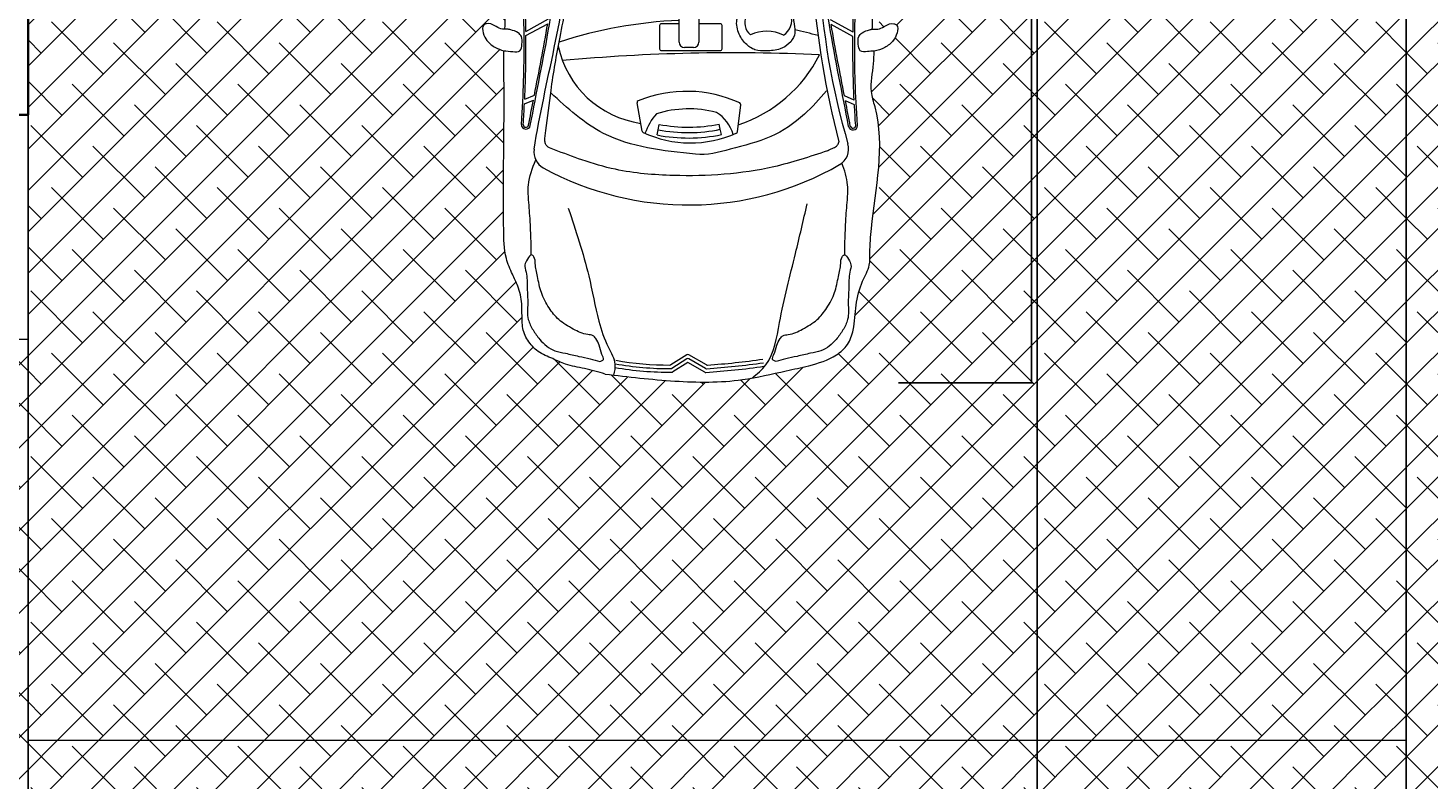
# Model space of a CAD drawing. Units: inches. Extents: x -4843 to -3402, y -164 to 3629.
# Tile 3 of 22: x -4303 to -3999, y 131 to 294. Entities that reach past the tile are written whole.
import ezdxf

# ---------------------------------------------------------------- set-up
doc = ezdxf.new("R2010")
doc.units = ezdxf.units.IN
for name, color, linetype, lineweight in [('A-ANNO-DIMS', 2, 'Continuous', 18), ('C-PRKG-VEHI', 7, 'Continuous', 18), ('C-PVMT', 7, 'Continuous', 18), ('walls', 7, 'Continuous', 35)]:
    doc.layers.add(name, color=color, linetype=linetype, lineweight=lineweight)
doc.layers.add('C-PVMT-PATT', color=9, linetype='Continuous', lineweight=13, true_color=0xc7c8ca)
doc.styles.get("Standard").update_dxf_attribs({"font": 'arial.ttf'})
doc.dimstyles.get("Standard").update_dxf_attribs({"dimtxt": 0.18, "dimasz": 0.18, "dimexe": 0.18, "dimexo": 0.0625, "dimgap": 0.09, "dimtad": 0, "dimtih": 1, "dimtoh": 1, "dimdec": 4, "dimzin": 0, "dimdsep": 46, "dimtxsty": 'Standard', "dimcen": 0.09, "dimadec": 0, "dimazin": 0, "dimtfac": 1, "dimtdec": 4, "dimtofl": 0, "dimtmove": 0, "dimatfit": 3, "dimfxl": 1, "dimtolj": 1, "dimtzin": 0, "dimarcsym": 0})
pattern_1 = [(45, (-7766.296, -1992.247), (-4.490128, 4.490128), []), (135, (-7766.296, -1992.247), (-13.470384, 4.490128), [15.875, -9.525])]

# ---------------------------------------------------------------- blocks, each defined once
blk = doc.blocks.new('A$C3DA776D3')
for p, q in [((1.3708, 1.8398), (1.39, 1.7957)), ((1.3941, 1.8386), (1.4148, 1.7908)), ((1.7076, 1.8326), (1.7664, 1.7249)), ((1.7285, 1.8328), (1.7896, 1.7211)), ((1.2367, 1.2599), (1.3767, 1.2842)), ((1.2178, 1.1855), (1.2439, 1.1804)), ((1.2439, 1.1804), (1.27, 1.1752)), ((0.0962, 1.0335), (0.0497, 1.1077)), ((0.114, 1.0384), (0.0674, 1.1128)), ((0.1347, 1.0387), (0.0852, 1.1179)), ((1.6488, 1.0062), (1.6488, 1.051)), ((1.6754, 1.0776), (1.84, 1.0776)), ((0.0487, 0.9511), (0.0962, 1.0335)), ((0.0668, 0.9469), (0.1142, 1.0292)), ((0.0848, 0.9427), (0.1349, 1.0296)), ((1.8376, 0.9796), (1.6754, 0.9796)), ((1.2197, 0.8688), (1.2457, 0.8743)), ((1.2457, 0.8743), (1.2717, 0.8798)), ((1.2339, 0.7901), (1.3663, 0.7728)), ((1.7032, 0.2201), (1.7621, 0.3277)), ((1.7242, 0.2199), (1.7853, 0.3316)), ((1.3665, 0.2129), (1.3856, 0.257)), ((1.3897, 0.2141), (1.4105, 0.2619))]:
    blk.add_line(p, q)
blk.add_lwpolyline([(1.7676, 0.9796), (1.7676, 0.876, -0.414214), (1.7587, 0.8671), (1.6411, 0.8671, -0.414214), (1.6323, 0.876), (1.6323, 1.1626, -0.414214), (1.6411, 1.1715), (1.7587, 1.1715, -0.414214), (1.7676, 1.1626), (1.7676, 1.0776)], format="xyb")
for centre, radius, start, end in [((1.2688, 1.8326), 0.0222, 88.30081, 259.23573), ((1.2688, 1.8326), 0.0133, 88.30081, 259.23573), ((2.3634, 1.0306), 1.4908, 151.27714, 209.97599), ((1.1337, 1.7044), 0.0887, 80.92793, 151.27714), ((1.7558, 1.1977), 0.4855, 101.85595, 171.84728), ((-0.4678, 0.9763), 2.2529, 2.57809, 17.91043), ((-7.7929, 0.8063), 9.4158, 357.43424, 5.15957), ((1.6427, 1.1201), 1.5944, 170.12112, 180.27968), ((1.6427, 1.1201), 1.5767, 170.06503, 180.09581), ((1.6427, 1.1201), 1.5589, 170.06503, 179.90871), ((1.7341, 1.0216), 0.5553, 155.15631, 204.0455), ((1.1185, 0.9515), 0.313, 49.40393, 69.93973), ((1.2382, 1.2512), 0.00887, 99.85481, 155.15631), ((0.8039, 1.0409), 0.6292, 335.29473, 22.22123), ((1.3782, 1.2755), 0.00887, 22.22123, 99.85481), ((1.9963, 1.0318), 0.7935, 168.82603, 191.84879), ((1.9963, 1.0318), 0.7669, 168.82603, 191.84879), ((1.9963, 1.0318), 0.7403, 168.82603, 191.84879), ((0.8099, 1.0292), 0.5366, 345.36448, 17.33436), ((0.0572, 1.1124), 0.00887, 180.27968, 212.03468), ((0.075, 1.1175), 0.00887, 180.09581, 212.03468), ((0.0927, 1.1226), 0.00887, 179.90871, 212.03468), ((0.1065, 1.0337), 0.00887, 330.07292, 32.03468), ((0.1272, 1.034), 0.00887, 330.07292, 32.03468), ((1.6754, 1.051), 0.0266, 90, 180), ((1.6754, 1.0062), 0.0266, 180, 270), ((0.0564, 0.9467), 0.00887, 150.07292, 183.67668), ((3.6022, 1.1745), 3.562, 183.67668, 188.32383), ((0.0745, 0.9425), 0.00887, 150.07292, 183.76336), ((3.6022, 1.1745), 3.5442, 183.76336, 188.32383), ((0.0925, 0.9383), 0.00887, 150.07292, 183.85072), ((3.6022, 1.1745), 3.5265, 183.85072, 188.32383), ((1.1715, 0.9872), 0.1833, 285.46201, 329.30509), ((1.235, 0.7989), 0.00887, 204.0455, 262.57695), ((1.9221, 0.9991), 0.6875, 198.09737, 243.3215), ((1.3675, 0.7816), 0.00887, 262.57695, 335.29473), ((1.5443, 0.6456), 0.1854, 333.48481, 25.53467), ((1.7703, 0.6782), 0.0753, 62.21447, 141.10294), ((1.782, 0.6059), 0.0837, 210.97226, 288.84464), ((-0.4678, 0.9763), 2.2529, 344.97, 347.97913), ((2.3306, -4.2069), 4.6409, 94.71361, 104.29398), ((2.1977, -3.2479), 3.6398, 93.02386, 106.34052), ((1.1488, 0.33), 0.0887, 209.97599, 286.34052), ((1.1826, 0.2989), 0.00887, 252.27428, 284.29398), ((1.2645, 0.2201), 0.0222, 100.76427, 271.69919), ((1.2645, 0.2201), 0.0133, 100.76427, 271.69919)]:
    blk.add_arc(centre, radius, start, end)
for points, knots in [([(1.633, 1.9421), (1.6372, 1.9559), (1.6485, 1.9865), (1.6785, 2.0254), (1.7174, 2.0443), (1.758, 2.0499), (1.7712, 2.0175), (1.7589, 1.9877), (1.737, 1.958), (1.7418, 1.929), (1.7342, 1.9007), (1.7274, 1.874), (1.7007, 1.849), (1.6682, 1.8516), (1.625, 1.8563), (1.6294, 1.9016), (1.6314, 1.9281), (1.633, 1.9421)], [0.0885943, 0.0885943, 0.0885943, 0.0885943, 0.1373899, 0.1989553, 0.2458559, 0.2904509, 0.3067594, 0.3537167, 0.3919221, 0.4272917, 0.447055, 0.4910496, 0.5184931, 0.5619515, 0.6001709, 0.6402891, 0.6890715, 0.6890715, 0.6890715, 0.6890715]), ([(0.0396, 1.4417), (0.0491, 1.4755), (0.0673, 1.5404), (0.0818, 1.6302), (0.1179, 1.7036), (0.1448, 1.7742), (0.1943, 1.8176), (0.2482, 1.8478), (0.3113, 1.8529), (0.3899, 1.8505), (0.4662, 1.8663), (0.5364, 1.9021), (0.6273, 1.9413), (0.825, 1.9427), (1.0734, 1.9431), (1.3668, 1.9392), (1.5418, 1.9411), (1.633, 1.9421)], [0, 0, 0, 0, 0.118823, 0.228347, 0.304709, 0.395218, 0.479661, 0.520666, 0.602694, 0.688012, 0.788383, 0.860898, 0.954729, 1.11959, 1.518327, 1.801929, 2.110556, 2.110556, 2.110556, 2.110556]), ([(1.7401, 1.9359), (1.7441, 1.9358), (1.8578, 1.931), (2.1105, 1.9445), (2.4984, 1.9427), (2.8874, 1.9396), (3.2079, 1.9402), (3.5092, 1.9401), (3.7388, 1.9191), (3.9196, 1.945), (3.9792, 1.9134), (4.0141, 1.8916), (4.0511, 1.8608), (4.0944, 1.8389), (4.1316, 1.8213), (4.1705, 1.8314), (4.2164, 1.8107), (4.2677, 1.7817), (4.3166, 1.7281), (4.3472, 1.6107), (4.3777, 1.4199), (4.3756, 1.126), (4.3499, 0.8209), (4.3562, 0.5655), (4.3432, 0.4036), (4.2994, 0.3183), (4.2485, 0.2679), (4.1835, 0.2317), (4.102, 0.2378), (4.0429, 0.19), (3.9911, 0.1682), (3.96, 0.1386), (3.7692, 0.1231), (3.5761, 0.125), (3.3929, 0.1252), (3.3707, 0.1253)], [0.114046, 0.114046, 0.114046, 0.114046, 0.127519, 0.499235, 0.968453, 1.440308, 1.814622, 2.054514, 2.455224, 2.610949, 2.635875, 2.681833, 2.750323, 2.797084, 2.847368, 2.883024, 2.926275, 3.011124, 3.084414, 3.16311, 3.41524, 3.739789, 4.152943, 4.449449, 4.607544, 4.693588, 4.767288, 4.84799, 4.936972, 5.028501, 5.093159, 5.12765, 5.168553, 5.718196, 5.794044, 5.794044, 5.794044, 5.794044]), ([(0.1019, 1.4686), (0.1062, 1.4841), (0.1156, 1.5181), (0.1267, 1.5748), (0.1418, 1.6322), (0.1526, 1.7039), (0.1991, 1.7596), (0.2557, 1.7978), (0.3143, 1.8295), (0.3862, 1.8206), (0.4642, 1.8281), (0.5263, 1.8249), (0.5774, 1.8421), (0.6026, 1.8255), (0.6352, 1.809), (0.6121, 1.7865), (0.5738, 1.7879), (0.515, 1.7735), (0.4383, 1.7603), (0.3668, 1.7216), (0.3014, 1.6709), (0.2619, 1.6015), (0.2328, 1.5457), (0.2321, 1.5021), (0.2099, 1.4834), (0.1779, 1.4679), (0.1449, 1.4643), (0.1093, 1.4427), (0.1042, 1.4606), (0.1019, 1.4686)], [0, 0, 0, 0, 0.048183, 0.105687, 0.173148, 0.226645, 0.320656, 0.377708, 0.433539, 0.514499, 0.587235, 0.668333, 0.704408, 0.73448, 0.764541, 0.77911, 0.812729, 0.87811, 0.959931, 1.044551, 1.119493, 1.20463, 1.28096, 1.307559, 1.326943, 1.363733, 1.411478, 1.437083, 1.45761, 1.45761, 1.45761, 1.45761]), ([(0.6291, 1.8062), (0.6836, 1.8072), (0.7737, 1.8088), (0.887, 1.8185), (0.9906, 1.8256), (1.0541, 1.8003), (1.0947, 1.7841)], [0, 0, 0, 0, 0.1633136, 0.269827, 0.3423859, 0.4712329, 0.4712329, 0.4712329, 0.4712329]), ([(1.2647, 1.8108), (1.5866, 1.75), (1.9321, 1.6711), (2.357, 1.6555), (2.4305, 1.6528), (2.5038, 1.6481)], [0.0116221, 0.0116221, 0.0116221, 0.0116221, 0.1543947, 0.1543947, 0.1841997, 0.1841997, 0.1841997, 0.1841997]), ([(1.2695, 1.8548), (1.4293, 1.844), (1.6772, 1.8374), (2.0858, 1.8517), (2.5501, 1.8477), (2.9741, 1.8297), (3.2389, 1.8174), (3.3308, 1.8077), (3.7511, 1.7597)], [0.04998, 0.04998, 0.04998, 0.04998, 0.456658, 0.88886, 1.432548, 2.02833, 2.31987, 2.336539, 2.336539, 2.336539, 2.336539]), ([(1.3941, 1.8386), (1.4513, 1.8358), (1.5039, 1.8341), (1.6065, 1.8322), (1.6573, 1.8322), (1.7076, 1.8326)], [0.1630874, 0.1630874, 0.1630874, 0.1630874, 0.3282058, 0.3282058, 0.4985864, 0.4985864, 0.4985864, 0.4985864]), ([(1.7285, 1.8328), (1.7747, 1.8334), (1.8206, 1.8343), (1.9706, 1.8377), (2.0741, 1.8401), (2.2558, 1.8407), (2.3339, 1.8401), (2.412, 1.8388)], [0.5222333, 0.5222333, 0.5222333, 0.5222333, 0.6789211, 0.6789211, 1.0296365, 1.0296365, 1.2940564, 1.2940564, 1.2940564, 1.2940564]), ([(1.1452, 1.6917), (1.1484, 1.7027), (1.1532, 1.7193), (1.17, 1.7359), (1.1994, 1.7411), (1.2882, 1.7262), (1.4597, 1.7082), (1.664, 1.6726), (1.8239, 1.6391), (1.9094, 1.627), (1.9434, 1.6262), (1.9633, 1.6236), (1.9429, 1.5472), (1.9237, 1.3694), (1.9156, 1.0748), (1.9104, 0.7612), (1.9305, 0.5688), (1.9526, 0.4525), (1.9572, 0.4288)], [0, 0, 0, 0, 0.038062, 0.057765, 0.075887, 0.136118, 0.360736, 0.660851, 0.833831, 0.919425, 0.944413, 0.95681, 0.976133, 1.15453, 1.659168, 1.908025, 2.226872, 2.308645, 2.308645, 2.308645, 2.308645]), ([(1.1477, 1.792), (1.4905, 1.7373), (1.7995, 1.6413), (2.2125, 1.6082), (2.2832, 1.6032), (2.2832, 1.6032)], [0.0003636, 0.0003636, 0.0003636, 0.0003636, 0.134701, 0.134701, 0.1508358, 0.1508358, 0.1508358, 0.1508358]), ([(1.1396, 0.3464), (1.1105, 0.4339), (1.0553, 0.5995), (1.019, 0.8559), (1.0138, 1.1174), (1.0332, 1.3547), (1.0902, 1.5485), (1.1279, 1.6467), (1.1452, 1.6917)], [0, 0, 0, 0, 0.276247, 0.522812, 0.772814, 1.060937, 1.232089, 1.37667, 1.37667, 1.37667, 1.37667]), ([(1.1227, 0.9968), (1.1398, 1.1559), (1.169, 1.4274), (1.3493, 1.6278), (1.4252, 1.7102)], [0, 0, 0, 0, 0.5236809, 0.8940297, 0.8940297, 0.8940297, 0.8940297]), ([(0.857, 1.6234), (0.7466, 1.5866), (0.5639, 1.5256), (0.3275, 1.4841), (0.1848, 1.438), (0.1003, 1.3859), (0.0525, 1.3961), (0.0346, 1.4)], [0, 0, 0, 0, 0.3490723, 0.577526, 0.7150863, 0.8038491, 0.8574249, 0.8574249, 0.8574249, 0.8574249]), ([(0.0396, 1.4417), (0.0259, 1.3277), (-0.001, 1.1032), (-0.0041, 0.801), (0.0486, 0.5837), (0.0809, 0.4273), (0.1148, 0.3191), (0.1818, 0.2415), (0.2711, 0.2106), (0.3792, 0.2096), (0.4873, 0.1821), (0.5671, 0.1351), (0.6573, 0.1377), (0.9147, 0.1185), (1.1883, 0.0534), (1.4506, 0.141), (1.5438, 0.1176), (1.6105, 0.116), (1.6314, 0.1164)], [0, 0, 0, 0, 0.388807, 0.765455, 1.01322, 1.141907, 1.30735, 1.390473, 1.477778, 1.61655, 1.755196, 1.851534, 1.920565, 2.05458, 2.731843, 2.819344, 2.97386, 3.044752, 3.044752, 3.044752, 3.044752]), ([(1.4353, 0.3505), (1.3953, 0.3854), (1.3056, 0.4639), (1.1968, 0.6245), (1.1532, 0.8126), (1.1151, 0.9395), (1.1227, 0.9968)], [0, 0, 0, 0, 0.1591256, 0.357512, 0.5668997, 0.7404451, 0.7404451, 0.7404451, 0.7404451]), ([(1.8119, 0.5169), (1.7917, 0.514), (1.7583, 0.5092), (1.7058, 0.5035), (1.6658, 0.5348), (1.6354, 0.5836), (1.6317, 0.6432), (1.632, 0.7046), (1.6686, 0.7545), (1.7219, 0.7885), (1.7812, 0.7994), (1.8082, 0.7822), (1.815, 0.7773)], [0, 0, 0, 0, 0.0697224, 0.1152553, 0.1718464, 0.228887, 0.3065165, 0.3695628, 0.4317857, 0.5044965, 0.584817, 0.6125638, 0.6125638, 0.6125638, 0.6125638]), ([(0.0196, 0.7177), (0.0398, 0.6931), (0.1079, 0.6118), (0.3423, 0.5784), (0.6005, 0.5098), (0.7967, 0.4646), (0.8786, 0.4458)], [0.006523, 0.006523, 0.006523, 0.006523, 0.111758, 0.359136, 0.754402, 1.03756, 1.03756, 1.03756, 1.03756]), ([(0.1019, 0.5984), (0.1062, 0.5829), (0.1156, 0.5489), (0.1267, 0.4922), (0.1418, 0.4348), (0.1526, 0.3631), (0.1991, 0.3074), (0.2557, 0.2692), (0.3143, 0.2375), (0.3862, 0.2464), (0.4642, 0.2389), (0.5263, 0.2421), (0.5774, 0.2249), (0.6026, 0.2415), (0.6352, 0.258), (0.6121, 0.2805), (0.5738, 0.2791), (0.515, 0.2935), (0.4383, 0.3067), (0.3668, 0.3454), (0.3014, 0.3961), (0.2619, 0.4655), (0.2328, 0.5213), (0.2321, 0.5649), (0.2099, 0.5836), (0.1779, 0.5991), (0.1449, 0.6027), (0.1093, 0.6243), (0.1042, 0.6063), (0.1019, 0.5984)], [0, 0, 0, 0, 0.048183, 0.105687, 0.173148, 0.226645, 0.320656, 0.377708, 0.433539, 0.514499, 0.587235, 0.668333, 0.704408, 0.73448, 0.764541, 0.77911, 0.812729, 0.87811, 0.959931, 1.044551, 1.119493, 1.20463, 1.28096, 1.307559, 1.326943, 1.363733, 1.411478, 1.437083, 1.45761, 1.45761, 1.45761, 1.45761]), ([(1.1396, 0.3464), (1.1438, 0.3385), (1.1517, 0.3239), (1.1594, 0.3017), (1.1724, 0.2931), (1.179, 0.2907), (1.1799, 0.2904)], [0, 0, 0, 0, 0.03043159, 0.05630154, 0.07707664, 0.0801121, 0.0801121, 0.0801121, 0.0801121]), ([(1.2603, 0.2419), (1.5822, 0.3027), (1.9277, 0.3816), (2.3526, 0.3972), (2.4261, 0.3999), (2.4995, 0.4046)], [0.0116221, 0.0116221, 0.0116221, 0.0116221, 0.1543947, 0.1543947, 0.1841997, 0.1841997, 0.1841997, 0.1841997]), ([(1.2651, 0.1979), (1.425, 0.2087), (1.6729, 0.2152), (2.0815, 0.2009), (2.5458, 0.205), (2.9697, 0.2229), (3.2345, 0.2353), (3.3264, 0.245), (3.7467, 0.293)], [0.04998, 0.04998, 0.04998, 0.04998, 0.456658, 0.88886, 1.432548, 2.02833, 2.31987, 2.336539, 2.336539, 2.336539, 2.336539]), ([(0.6291, 0.2608), (0.6836, 0.2598), (0.7736, 0.2582), (0.887, 0.2484), (0.9849, 0.2419), (1.0439, 0.2621), (1.0797, 0.2744)], [0, 0, 0, 0, 0.1633136, 0.269827, 0.3423859, 0.4544922, 0.4544922, 0.4544922, 0.4544922]), ([(1.3897, 0.2141), (1.447, 0.2169), (1.4995, 0.2186), (1.6021, 0.2205), (1.6529, 0.2205), (1.7032, 0.2201)], [0.1630874, 0.1630874, 0.1630874, 0.1630874, 0.3282058, 0.3282058, 0.4985864, 0.4985864, 0.4985864, 0.4985864]), ([(1.7242, 0.2199), (1.7704, 0.2193), (1.8163, 0.2184), (1.9663, 0.215), (2.0698, 0.2126), (2.2514, 0.212), (2.3295, 0.2126), (2.4077, 0.2138)], [0.5222333, 0.5222333, 0.5222333, 0.5222333, 0.6789211, 0.6789211, 1.0296365, 1.0296365, 1.2940564, 1.2940564, 1.2940564, 1.2940564]), ([(1.6314, 0.1164), (1.6344, 0.0983), (1.6457, 0.0631), (1.6785, 0.0206), (1.7174, 0.0016), (1.758, -0.0039), (1.7712, 0.0285), (1.7589, 0.0583), (1.737, 0.0879), (1.7418, 0.117), (1.7342, 0.1453), (1.7274, 0.1719), (1.7007, 0.197), (1.6682, 0.1944), (1.625, 0.1897), (1.6289, 0.1495), (1.6307, 0.1265), (1.6314, 0.1164)], [0.0739443, 0.0739443, 0.0739443, 0.0739443, 0.1373899, 0.1989553, 0.2458559, 0.2904509, 0.3067594, 0.3537167, 0.3919221, 0.4272917, 0.447055, 0.4910496, 0.5184931, 0.5619515, 0.6001709, 0.6402891, 0.6746905, 0.6746905, 0.6746905, 0.6746905])]:
    blk.add_open_spline(points, degree=3, knots=knots)
for points in [[(1.2663, 1.8195), (1.3072, 1.8118), (1.3484, 1.8038), (1.39, 1.7957)], [(1.2689, 1.8459), (1.3047, 1.8435), (1.3385, 1.8415), (1.3708, 1.8398)], [(1.4148, 1.7908), (1.5298, 1.7683), (1.6473, 1.7451), (1.7664, 1.7249)], [(1.4105, 0.2619), (1.5255, 0.2844), (1.6429, 0.3076), (1.7621, 0.3277)], [(1.262, 0.2332), (1.3028, 0.2409), (1.3441, 0.2489), (1.3856, 0.257)], [(1.2645, 0.2068), (1.3003, 0.2092), (1.3342, 0.2112), (1.3665, 0.2129)], [(1.7393, 0.1245), (1.7407, 0.1247), (1.7421, 0.1248), (1.7436, 0.125)], [(2.2804, 0.1218), (2.1011, 0.1222), (1.9224, 0.1236), (1.7436, 0.125)]]:
    blk.add_open_spline(points, degree=3)
blk = doc.blocks.new('*D58')
at = {"layer": 'A-ANNO-DIMS', "color": 0, "lineweight": -2, "transparency": 16777216}
for p, q in [((-4113.85, 410.04), (-4084.81, 410.04)), ((-4084.99, 409.86), (-4084.99, 313.81)), ((-4084.99, 217.38), (-4084.99, 313.44)), ((-4113.85, 217.2), (-4084.81, 217.2))]:
    blk.add_line(p, q, dxfattribs=at)
at = {"layer": 'A-ANNO-DIMS', "color": 0, "transparency": 16777216}
for points in [[(-4085.02, 409.86), (-4084.96, 409.86), (-4084.99, 410.04)], [(-4085.02, 217.38), (-4084.96, 217.38), (-4084.99, 217.2)]]:
    blk.add_solid(points, dxfattribs=at)
at = {"layer": 'Defpoints', "color": 0, "transparency": 16777216}
for p in [(-4113.92, 410.04), (-4084.99, 410.04), (-4113.92, 217.2)]:
    blk.add_point(p, dxfattribs=at)
at = {"layer": 'A-ANNO-DIMS', "color": 0, "transparency": 16777216, "insert": (-4084.99, 313.62), "char_height": 0.18, "attachment_point": 5}
blk.add_mtext('\\A1;CAR 193', dxfattribs=at)
blk = doc.blocks.new('*D63')
at = {"layer": 'A-ANNO-DIMS', "color": 0, "lineweight": -2, "transparency": 16777216}
for p, q in [((-4083.78, 457.29), (-4083.78, 10.92)), ((-4302.78, 275.29), (-4302.78, 10.92)), ((-4302.6, 11.1), (-4193.57, 11.1)), ((-4083.96, 11.1), (-4192.99, 11.1))]:
    blk.add_line(p, q, dxfattribs=at)
at = {"layer": 'A-ANNO-DIMS', "color": 0, "transparency": 16777216}
for points in [[(-4302.6, 11.13), (-4302.6, 11.07), (-4302.78, 11.1)], [(-4083.96, 11.13), (-4083.96, 11.07), (-4083.78, 11.1)]]:
    blk.add_solid(points, dxfattribs=at)
at = {"layer": 'Defpoints', "color": 0, "transparency": 16777216}
for p in [(-4083.78, 457.35), (-4302.78, 275.35), (-4083.78, 11.1)]:
    blk.add_point(p, dxfattribs=at)
at = {"layer": 'A-ANNO-DIMS', "color": 0, "transparency": 16777216, "insert": (-4193.28, 11.1), "char_height": 0.18, "attachment_point": 5}
blk.add_mtext('\\A1;219', dxfattribs=at)
blk = doc.blocks.new('*D66')
at = {"layer": 'A-ANNO-DIMS', "color": 0, "lineweight": -2, "transparency": 16777216}
for p, q in [((-4083.78, 457.29), (-4083.78, 10.92)), ((-3941.78, 86.29), (-3941.78, 10.92)), ((-4083.6, 11.1), (-4013.06, 11.1)), ((-3941.96, 11.1), (-4012.5, 11.1))]:
    blk.add_line(p, q, dxfattribs=at)
at = {"layer": 'A-ANNO-DIMS', "color": 0, "transparency": 16777216}
for points in [[(-4083.6, 11.13), (-4083.6, 11.07), (-4083.78, 11.1)], [(-3941.96, 11.13), (-3941.96, 11.07), (-3941.78, 11.1)]]:
    blk.add_solid(points, dxfattribs=at)
at = {"layer": 'Defpoints', "color": 0, "transparency": 16777216}
for p in [(-4083.78, 457.35), (-3941.78, 86.35), (-3941.78, 11.1)]:
    blk.add_point(p, dxfattribs=at)
at = {"layer": 'A-ANNO-DIMS', "color": 0, "transparency": 16777216, "insert": (-4012.78, 11.1), "char_height": 0.18, "attachment_point": 5}
blk.add_mtext('\\A1;142', dxfattribs=at)
blk = doc.blocks.new('*D81')
at = {"layer": 'A-ANNO-DIMS', "color": 0, "lineweight": -2, "transparency": 16777216}
for p, q in [((-4332.78, 86.42), (-4332.78, 1392.95)), ((-4332.6, 1392.77), (-4168.61, 1392.77)), ((-4003.86, 1392.77), (-4167.86, 1392.77)), ((-4003.68, 86.42), (-4003.68, 1392.95))]:
    blk.add_line(p, q, dxfattribs=at)
at = {"layer": 'A-ANNO-DIMS', "color": 0, "transparency": 16777216}
for points in [[(-4332.6, 1392.8), (-4332.6, 1392.74), (-4332.78, 1392.77)], [(-4003.86, 1392.8), (-4003.86, 1392.74), (-4003.68, 1392.77)]]:
    blk.add_solid(points, dxfattribs=at)
at = {"layer": 'Defpoints', "color": 0, "transparency": 16777216}
for p in [(-4003.68, 1392.77), (-4332.78, 86.35), (-4003.68, 86.35)]:
    blk.add_point(p, dxfattribs=at)
at = {"layer": 'A-ANNO-DIMS', "color": 0, "transparency": 16777216, "insert": (-4168.23, 1392.77), "char_height": 0.18, "attachment_point": 5}
blk.add_mtext('\\A1;329.1', dxfattribs=at)

msp = doc.modelspace()

# ---------------------------------------------------------------- hatches: boundary and pattern name
at = {"layer": 'C-PVMT-PATT'}
h = msp.add_hatch(dxfattribs=at)
h.set_pattern_fill('ANSI38', color=256, scale=2)
h.set_pattern_definition(pattern_1)
h.paths.add_polyline_path([(-4583.98, 275.35), (-4595.78, 275.35), (-4595.78, 324.35), (-4595.78, 373.35), (-4595.78, 466.35), (-4696.78, 466.35), (-4696.78, 95.35), (-4583.98, 95.35), (-4583.98, 226.6)])
h.paths.add_polyline_path([(-4302.78, 226.6), (-4583.98, 226.6), (-4583.98, 95.35), (-4332.78, 95.35), (-4332.78, 86.35), (-4003.68, 86.35), (-4003.68, 95.35), (-3978.78, 95.35), (-3978.78, 457.35), (-4003.68, 457.35), (-4003.68, 139.54), (-4302.78, 139.54)])
h = msp.add_hatch(dxfattribs=at)
h.set_pattern_fill('ANSI38', color=256, scale=2)
h.set_pattern_definition(pattern_1)
h.paths.add_polyline_path([(-4302.78, 139.54), (-4003.68, 139.54), (-4003.68, 457.35), (-4302.78, 457.35)])
edge = h.paths.add_edge_path(flags=16)
edge.add_spline(control_points=[(-4177.52, 219.09), (-4179, 219.51), (-4181.86, 220.31), (-4185.82, 220.95), (-4189.05, 222.54), (-4192.16, 223.72), (-4194.07, 225.9), (-4195.4, 228.28), (-4195.62, 231.06), (-4195.51, 234.52), (-4196.21, 237.87), (-4197.78, 240.97), (-4199.51, 244.96), (-4199.58, 253.67), (-4199.59, 264.61), (-4199.42, 277.52), (-4199.5, 285.22), (-4199.55, 289.24)], knot_values=[0, 0, 0, 0, 0.118823, 0.228347, 0.304709, 0.395218, 0.479661, 0.520666, 0.602694, 0.688012, 0.788383, 0.860898, 0.954729, 1.11959, 1.518327, 1.801929, 2.110556, 2.110556, 2.110556, 2.110556], degree=3, periodic=0)
edge.add_spline(control_points=[(-4199.55, 289.24), (-4200.15, 289.43), (-4201.5, 289.92), (-4203.22, 291.24), (-4204.05, 292.95), (-4204.29, 294.74), (-4202.87, 295.32), (-4201.55, 294.78), (-4200.39, 293.92), (-4199.58, 293.95), (-4199.28, 293.95)], knot_values=[0.088594, 0.088594, 0.088594, 0.088594, 0.13739, 0.198955, 0.245856, 0.290451, 0.306759, 0.353717, 0.391922, 0.414753, 0.414753, 0.414753, 0.414753], degree=3, periodic=0)
edge.add_spline(control_points=[(-4199.28, 293.95), (-4199.27, 294.13), (-4199.06, 299.13), (-4199.65, 310.26), (-4199.6, 321.33), (-4199.56, 327.57), (-4199.56, 327.7)], knot_values=[0.114046, 0.114046, 0.114046, 0.114046, 0.127519, 0.499235, 0.968453, 0.97871, 0.97871, 0.97871, 0.97871], degree=3, periodic=0)
edge.add_spline(control_points=[(-4199.56, 327.7), (-4199.52, 333.71), (-4199.44, 344.59), (-4199.46, 358.57), (-4199.46, 371.83), (-4198.54, 381.94), (-4199.67, 389.9), (-4198.28, 392.53), (-4197.33, 394.06), (-4195.97, 395.69), (-4195, 397.6), (-4194.23, 399.23), (-4194.68, 400.94), (-4193.76, 402.97), (-4192.49, 405.22), (-4190.13, 407.38), (-4184.96, 408.73), (-4176.56, 410.07), (-4163.62, 409.97), (-4150.19, 408.84), (-4138.94, 409.12), (-4131.82, 408.55), (-4128.06, 406.62), (-4125.85, 404.38), (-4124.25, 401.52), (-4124.52, 397.93), (-4122.42, 395.33), (-4121.46, 393.05), (-4120.15, 391.68), (-4119.47, 383.28), (-4119.55, 374.78), (-4119.57, 366.71), (-4119.57, 365.74)], knot_values=[0.97871, 0.97871, 0.97871, 0.97871, 1.440308, 1.814622, 2.054514, 2.455224, 2.610949, 2.635875, 2.681833, 2.750323, 2.797084, 2.847368, 2.883024, 2.926275, 3.011124, 3.084414, 3.16311, 3.41524, 3.739789, 4.152943, 4.449449, 4.607544, 4.693588, 4.767288, 4.84799, 4.936972, 5.028501, 5.093159, 5.12765, 5.168553, 5.718196, 5.794044, 5.794044, 5.794044, 5.794044], degree=3, periodic=0)
edge.add_spline(control_points=[(-4120.18, 367.25), (-4120.14, 367.18), (-4119.97, 366.93), (-4119.55, 366.17), (-4119.49, 364.82), (-4119.6, 363.39), (-4120.03, 362.65), (-4120.18, 362.38)], knot_values=[0, 0, 0, 0, 0.00069, 0.002823, 0.007863, 0.012889, 0.015703, 0.015703, 0.015703, 0.015703], degree=3, periodic=0)
edge.add_spline(control_points=[(-4119.57, 364.08), (-4119.56, 351.01), (-4119.42, 337.76), (-4119.41, 324.56)], knot_values=[5.836848, 5.836848, 5.836848, 5.836848, 6.848265, 6.848265, 6.848265, 6.848265], degree=3, periodic=0)
edge.add_ellipse((-4119.53, 321.37), major_axis=(-0.07, 3.66), ratio=0.102782, start_angle=-179.3184, end_angle=-3.3021, ccw=False)
edge.add_spline(control_points=[(-4119.41, 317.74), (-4119.43, 309.85), (-4119.49, 301.98), (-4119.55, 294.11)], knot_values=[7.022686, 7.022686, 7.022686, 7.022686, 7.62832, 7.62832, 7.62832, 7.62832], degree=3, periodic=0)
edge.add_spline(control_points=[(-4119.55, 294.11), (-4119.55, 294.04), (-4119.54, 293.98), (-4119.53, 293.92)], knot_values=[3.166598, 3.166598, 3.166598, 3.166598, 3.17144, 3.17144, 3.17144, 3.17144], degree=3, periodic=0)
edge.add_spline(control_points=[(-4119.53, 293.92), (-4119.49, 293.93), (-4118.98, 293.99), (-4117.92, 293.82), (-4116.62, 294.78), (-4115.3, 295.32), (-4113.88, 294.74), (-4114.12, 292.95), (-4114.96, 291.24), (-4116.83, 289.8), (-4118.38, 289.3), (-4119.18, 289.17)], knot_values=[0.073944, 0.073944, 0.073944, 0.073944, 0.077675, 0.113045, 0.15125, 0.198208, 0.214516, 0.259111, 0.306012, 0.367577, 0.431023, 0.431023, 0.431023, 0.431023], degree=3, periodic=0)
edge.add_spline(control_points=[(-4119.18, 289.17), (-4119.16, 288.25), (-4119.23, 285.31), (-4120.26, 281.21), (-4116.4, 269.66), (-4119.27, 257.62), (-4120.12, 246.29), (-4120, 242.31), (-4122.07, 238.8), (-4123.28, 234.04), (-4123.32, 229.29), (-4124.68, 225.36), (-4128.1, 222.41), (-4132.86, 220.91), (-4139.06, 219.63), (-4143.16, 218.66), (-4145.64, 218.22)], knot_values=[0.819302, 0.819302, 0.819302, 0.819302, 0.890194, 1.044711, 1.132212, 1.809474, 1.943489, 2.01252, 2.108859, 2.247504, 2.386276, 2.473581, 2.556705, 2.722147, 2.850835, 3.044752, 3.044752, 3.044752, 3.044752], degree=3, periodic=0)
edge.add_spline(control_points=[(-4145.64, 218.22), (-4146.33, 218.09), (-4151.86, 217.2), (-4162, 217.3), (-4171.27, 218.35), (-4175.68, 218.87)], knot_values=[0.047426, 0.047426, 0.047426, 0.047426, 0.101273, 0.477921, 0.819302, 0.819302, 0.819302, 0.819302], degree=3, periodic=0)
edge.add_spline(control_points=[(-4175.68, 218.87), (-4176.29, 218.95), (-4176.91, 219.02), (-4177.52, 219.09)], knot_values=[0, 0, 0, 0, 0.047426, 0.047426, 0.047426, 0.047426], degree=3, periodic=0)
edge = h.paths.add_edge_path(flags=0)
edge.add_spline(control_points=[(-4193.77, 273.03), (-4191.09, 287.2), (-4187.62, 302.4), (-4186.93, 321.11), (-4186.81, 324.35), (-4186.61, 327.58)], knot_values=[0.011622, 0.011622, 0.011622, 0.011622, 0.154395, 0.154395, 0.1842, 0.1842, 0.1842, 0.1842], degree=3, periodic=0)
edge.add_arc((-14109, 562.63), 9925.18, 358.64295, 358.862544)
edge.add_arc((-4243.78, 366.9), 58.02, 358.7216, 381.1082)
edge.add_arc((-4190.02, 387.65), 0.39, 21.1082, 164.1707)
edge.add_arc((-4151.78, 376.81), 40.14, 164.1707, 171.876)
edge.add_spline(control_points=[(-4191.52, 382.48), (-4193.63, 363.98), (-4194.06, 359.93), (-4194.6, 348.28), (-4195.39, 329.61), (-4195.57, 309.17), (-4194.94, 291.19), (-4195.23, 280.27), (-4195.7, 273.24)], knot_values=[0.04998, 0.04998, 0.04998, 0.04998, 0.066649, 0.35819, 0.953971, 1.497659, 1.929861, 2.336539, 2.336539, 2.336539, 2.336539], degree=3, periodic=0)
edge.add_arc((-4194.73, 273.21), 0.976, 178.3008, 349.1958)
edge = h.paths.add_edge_path(flags=0)
edge.add_spline(control_points=[(-4195.31, 273.22), (-4195.21, 274.79), (-4195.12, 276.28), (-4195.04, 277.7)], knot_values=[0.050139, 0.050139, 0.050139, 0.050139, 0.140986, 0.140986, 0.140986, 0.140986], degree=3, periodic=0)
edge.add_line((-4195.04, 277.7), (-4193.1, 278.54))
edge.add_spline(control_points=[(-4193.1, 278.54), (-4193.46, 276.71), (-4193.81, 274.9), (-4194.15, 273.1)], knot_values=[0.011622, 0.011622, 0.011622, 0.011622, 0.029731, 0.029731, 0.029731, 0.029731], degree=3, periodic=0)
edge.add_arc((-4194.73, 273.21), 0.586, 178.9277, 349.1656, ccw=False)
edge = h.paths.add_edge_path(flags=0)
edge.add_spline(control_points=[(-4192.94, 267.88), (-4190.53, 282.97), (-4186.3, 296.57), (-4184.85, 314.75), (-4184.63, 317.86), (-4184.63, 317.86)], knot_values=[0.000364, 0.000364, 0.000364, 0.000364, 0.134701, 0.134701, 0.150836, 0.150836, 0.150836, 0.150836], degree=3, periodic=0)
edge.add_spline(control_points=[(-4184.63, 317.86), (-4184.48, 319.61), (-4184.14, 329.7), (-4184.58, 344.88), (-4184.71, 357.85), (-4185.28, 371.27)], knot_values=[0.036478, 0.036478, 0.036478, 0.036478, 0.053439, 0.129277, 0.173634, 0.173634, 0.173634, 0.173634], degree=3, periodic=0)
edge.add_arc((-4181.38, 371.43), 3.9, 95.3633, 182.3534, ccw=False)
edge.add_spline(control_points=[(-4181.75, 375.32), (-4178.43, 375.63), (-4172.02, 376.65), (-4161.57, 377.87), (-4149.14, 377.13), (-4140.59, 376.64), (-4136.44, 375.2)], knot_values=[0.007384, 0.007384, 0.007384, 0.007384, 0.029401, 0.067193, 0.103796, 0.144479, 0.144479, 0.144479, 0.144479], degree=3, periodic=0)
edge.add_arc((-4137.72, 371.51), 3.9, -1.298, 70.8366, ccw=False)
edge.add_spline(control_points=[(-4133.81, 371.42), (-4133.92, 366.8), (-4133.8, 365.25), (-4134.1, 356.56), (-4133.51, 346.62), (-4132.74, 328.68), (-4132.62, 320.9), (-4131.51, 309.76), (-4131.36, 307.85), (-4131.08, 305.65)], knot_values=[0.107006, 0.107006, 0.107006, 0.107006, 0.118332, 0.118332, 0.206466, 0.206466, 0.276418, 0.276418, 0.309317, 0.309317, 0.309317, 0.309317], degree=3, periodic=0)
edge.add_arc((-3971.07, 314.1), 160.23, 183.0239, 196.3405)
edge.add_arc((-4128.58, 267.92), 3.9, -60.024, 16.3405, ccw=False)
edge.add_arc((-4159.42, 321.39), 65.63, 241.2771, 299.976, ccw=False)
edge.add_arc((-4189.08, 267.26), 3.9, 170.9279, 241.2771, ccw=False)
edge = h.paths.add_edge_path(flags=0)
edge.add_spline(control_points=[(-4194.99, 278.72), (-4194.87, 281.24), (-4194.79, 283.56), (-4194.71, 288.07), (-4194.71, 290.31), (-4194.73, 292.52)], knot_values=[0.163087, 0.163087, 0.163087, 0.163087, 0.328206, 0.328206, 0.498586, 0.498586, 0.498586, 0.498586], degree=3, periodic=0)
edge.add_line((-4194.73, 292.52), (-4189.99, 295.11))
edge.add_spline(control_points=[(-4189.99, 295.11), (-4190.88, 289.87), (-4191.9, 284.7), (-4192.89, 279.64)], knot_values=[0.033336, 0.033336, 0.033336, 0.033336, 0.083278, 0.083278, 0.083278, 0.083278], degree=3, periodic=0)
edge.add_line((-4192.89, 279.64), (-4194.99, 278.72))
edge = h.paths.add_edge_path(flags=0)
edge.add_spline(control_points=[(-4178.7, 221.84), (-4179.39, 222.03), (-4180.88, 222.44), (-4183.38, 222.93), (-4185.9, 223.59), (-4189.06, 224.07), (-4191.51, 226.12), (-4193.19, 228.61), (-4194.59, 231.18), (-4194.2, 234.35), (-4194.53, 237.78), (-4194.39, 240.52), (-4195.15, 242.77), (-4194.42, 243.88), (-4193.69, 245.31), (-4192.7, 244.3), (-4192.76, 242.61), (-4192.13, 240.02), (-4191.54, 236.65), (-4189.84, 233.5), (-4187.61, 230.62), (-4184.55, 228.88), (-4182.1, 227.6), (-4180.18, 227.57), (-4179.35, 226.59), (-4178.67, 225.18), (-4178.52, 223.73), (-4177.56, 222.16), (-4178.35, 221.94), (-4178.7, 221.84)], knot_values=[0, 0, 0, 0, 0.048183, 0.105687, 0.173148, 0.226645, 0.320656, 0.377708, 0.433539, 0.514499, 0.587235, 0.668333, 0.704408, 0.73448, 0.764541, 0.77911, 0.812729, 0.87811, 0.959931, 1.044551, 1.119493, 1.20463, 1.28096, 1.307559, 1.326943, 1.363733, 1.411478, 1.437083, 1.45761, 1.45761, 1.45761, 1.45761], degree=3, periodic=0)
edge = h.paths.add_edge_path(flags=0)
edge.add_spline(control_points=[(-4188.52, 267.77), (-4189.01, 267.9), (-4189.74, 268.12), (-4190.47, 268.86), (-4190.7, 270.15), (-4190.08, 273.88), (-4189.7, 277.37), (-4189.34, 280.09)], knot_values=[0, 0, 0, 0, 0.038062, 0.057765, 0.075887, 0.136118, 0.346676, 0.346676, 0.346676, 0.346676], degree=3, periodic=0)
edge.add_spline(control_points=[(-4189.34, 280.09), (-4189.32, 280.27), (-4188.86, 283.67), (-4188.3, 287.07), (-4187.7, 290.25)], knot_values=[0.346676, 0.346676, 0.346676, 0.346676, 0.360736, 0.61029, 0.61029, 0.61029, 0.61029], degree=3, periodic=0)
edge.add_spline(control_points=[(-4187.7, 290.25), (-4187.64, 290.55), (-4187.59, 290.84), (-4187.53, 291.13)], knot_values=[0.61029, 0.61029, 0.61029, 0.61029, 0.63318, 0.63318, 0.63318, 0.63318], degree=3, periodic=0)
edge.add_spline(control_points=[(-4187.53, 291.13), (-4187.46, 291.48), (-4186.97, 294.04), (-4186.21, 297.64), (-4185.68, 301.41), (-4185.64, 302.9), (-4185.53, 303.78), (-4182.16, 302.88), (-4174.34, 302.04), (-4164.13, 301.75), (-4156.84, 301.61), (-4156.19, 301.6)], knot_values=[0.63318, 0.63318, 0.63318, 0.63318, 0.660851, 0.833831, 0.919425, 0.944413, 0.95681, 0.976133, 1.15453, 1.659168, 1.709179, 1.709179, 1.709179, 1.709179], degree=3, periodic=0)
edge.add_spline(control_points=[(-4156.19, 301.6), (-4155.1, 301.58), (-4154.03, 301.57), (-4152.95, 301.57)], knot_values=[1.709179, 1.709179, 1.709179, 1.709179, 1.79199, 1.79199, 1.79199, 1.79199], degree=3, periodic=0)
edge.add_spline(control_points=[(-4152.95, 301.57), (-4152.42, 301.57), (-4151.9, 301.57), (-4151.37, 301.57)], knot_values=[1.79199, 1.79199, 1.79199, 1.79199, 1.832683, 1.832683, 1.832683, 1.832683], degree=3, periodic=0)
edge.add_spline(control_points=[(-4151.37, 301.57), (-4150.4, 301.58), (-4145.3, 301.69), (-4139.09, 302.34), (-4133.97, 303.31), (-4132.93, 303.51)], knot_values=[1.832683, 1.832683, 1.832683, 1.832683, 1.908025, 2.226872, 2.308645, 2.308645, 2.308645, 2.308645], degree=3, periodic=0)
edge.add_arc((-4132.85, 303.13), 0.39, 4.7136, 100.9875, ccw=False)
edge.add_arc((-3928.85, 319.95), 204.3, 184.7136, 194.294)
edge.add_arc((-4127.21, 269.41), 0.39, -17.7257, 14.294, ccw=False)
edge.add_spline(control_points=[(-4126.84, 269.29), (-4126.85, 269.25), (-4126.95, 268.96), (-4127.33, 268.39), (-4128.31, 268.05), (-4128.95, 267.71), (-4129.3, 267.52)], knot_values=[0, 0, 0, 0, 0.003035, 0.023811, 0.049681, 0.080112, 0.080112, 0.080112, 0.080112], degree=3, periodic=0)
edge.add_spline(control_points=[(-4129.3, 267.52), (-4133.15, 266.24), (-4140.45, 263.81), (-4151.73, 262.21), (-4163.24, 261.98), (-4173.69, 262.83), (-4182.22, 265.35), (-4186.54, 267.01), (-4188.52, 267.77)], knot_values=[0, 0, 0, 0, 0.276247, 0.522812, 0.772814, 1.060937, 1.232089, 1.37667, 1.37667, 1.37667, 1.37667], degree=3, periodic=0)
edge = h.paths.add_edge_path(flags=0)
edge.add_spline(control_points=[(-4194.74, 293.44), (-4194.76, 295.48), (-4194.8, 297.5), (-4194.95, 304.1), (-4195.06, 308.66), (-4195.08, 316.65), (-4195.06, 320.09), (-4195, 323.53)], knot_values=[0.522233, 0.522233, 0.522233, 0.522233, 0.678921, 0.678921, 1.029636, 1.029636, 1.294056, 1.294056, 1.294056, 1.294056], degree=3, periodic=0)
edge.add_arc((-4194.61, 323.53), 0.39, 118.6584, 180.1243, ccw=False)
edge.add_line((-4194.8, 323.87), (-4187.58, 327.81))
edge.add_arc((-4187.4, 327.47), 0.39, -1.7955, 118.6584, ccw=False)
edge.add_spline(control_points=[(-4187.01, 327.45), (-4187.19, 324.61), (-4187.3, 321.78), (-4187.57, 314.47), (-4187.91, 310.04), (-4188.83, 302.44), (-4189.3, 299.28), (-4189.82, 296.13)], knot_values=[0.086512, 0.086512, 0.086512, 0.086512, 0.1126, 0.1126, 0.153879, 0.153879, 0.183727, 0.183727, 0.183727, 0.183727], degree=3, periodic=0)
edge.add_line((-4189.82, 296.13), (-4194.74, 293.44))
h.paths.add_polyline_path([(-4186.78, 287.12, -0.033695), (-4130.99, 288.38, -0.199929), (-4148.63, 273.2), (-4148.83, 271.67, -0.261093), (-4149.06, 271.36, -0.216615), (-4169.29, 271.5, -0.246093), (-4169.52, 271.79), (-4169.81, 273.49, -0.273701)], flags=0)
edge = h.paths.add_edge_path(flags=0)
edge.add_arc((-4140.72, 295.8), 3.69, -59.0277, 20.0091, ccw=False)
edge.add_arc((-4142.47, 285.34), 8.16, 63.4848, 115.5347)
edge.add_arc((-4143.91, 295.28), 3.32, 152.2145, 231.1029, ccw=False)
edge.add_ellipse((-4142.44, 301.89), major_axis=(10.53, 0), ratio=0.529672, start_angle=218.5261, end_angle=229.0127, ccw=False)
edge.add_spline(control_points=[(-4148.27, 297.25), (-4148.49, 296.95), (-4148.81, 296.44), (-4148.95, 295.85), (-4148.97, 295.61)], knot_values=[0.565799, 0.565799, 0.565799, 0.565799, 0.593545, 0.612564, 0.612564, 0.612564, 0.612564], degree=3, periodic=0)
edge.add_spline(control_points=[(-4148.97, 295.61), (-4149.06, 294.82), (-4148.63, 292.94), (-4147.27, 290.81), (-4145.07, 289.2), (-4142.36, 289.18), (-4139.75, 289.34), (-4137.6, 290.68), (-4136.36, 292.26), (-4136.35, 293.38), (-4136.37, 293.76)], knot_values=[0.086242, 0.086242, 0.086242, 0.086242, 0.147544, 0.220255, 0.282478, 0.345524, 0.423154, 0.480194, 0.536785, 0.565799, 0.565799, 0.565799, 0.565799], degree=3, periodic=0)
edge.add_spline(control_points=[(-4136.37, 293.76), (-4136.39, 293.98), (-4136.52, 295.13), (-4136.68, 296.22), (-4136.81, 297.11)], knot_values=[0, 0, 0, 0, 0.016519, 0.086242, 0.086242, 0.086242, 0.086242], degree=3, periodic=0)
edge.add_ellipse((-4142.44, 301.89), major_axis=(10.53, 0), ratio=0.529672, start_angle=229.0127, end_angle=352.38, ccw=False)
edge = h.paths.add_edge_path(flags=0)
edge.add_ellipse((-4159.28, 300.8), major_axis=(0, 3.41), ratio=0.932272, start_angle=137.9206, end_angle=219.4265)
edge.add_line((-4157.17, 298.24), (-4157.17, 295.16))
edge.add_line((-4157.17, 295.16), (-4152.61, 295.16))
edge.add_arc((-4152.61, 294.77), 0.39, 0, 90, ccw=False)
edge.add_line((-4152.22, 294.77), (-4152.22, 289.6))
edge.add_arc((-4152.61, 289.6), 0.39, -90, 0, ccw=False)
edge.add_line((-4152.61, 289.21), (-4165.23, 289.21))
edge.add_arc((-4165.23, 289.6), 0.39, 180, 270, ccw=False)
edge.add_line((-4165.62, 289.6), (-4165.62, 294.77))
edge.add_arc((-4165.23, 294.77), 0.39, 90, 180, ccw=False)
edge.add_line((-4165.23, 295.16), (-4161.49, 295.16))
edge.add_line((-4161.49, 295.16), (-4161.49, 298.35))
edge = h.paths.add_edge_path(flags=0)
edge.add_ellipse((-4198.94, 321.56), major_axis=(0.07, 3.66), ratio=0.102782, start_angle=0, end_angle=360)

# ---------------------------------------------------------------- linework, layer by layer
at = {"layer": 'C-PVMT'}
msp.add_lwpolyline([(-4302.78, 457.35), (-4003.68, 457.35), (-4003.68, 139.54), (-4302.78, 139.54)], close=True, dxfattribs=at)
msp.add_lwpolyline([(-4583.63, 275.35), (-4302.78, 275.35), (-4302.78, 226.6), (-4583.98, 226.6)], dxfattribs=at)
at = {"layer": 'walls'}
for p, q in [((-4302.78, 457.35), (-4302.78, 275.35)), ((-4302.78, 275.35), (-4320.78, 275.35))]:
    msp.add_line(p, q, dxfattribs=at)

# ---------------------------------------------------------------- block references
at = {"layer": 'C-PRKG-VEHI', "xscale": 44.02240072481096, "yscale": 44.02240072481096, "zscale": 44.02240072481096, "rotation": 90}
msp.add_blockref('A$C3DA776D3', (-4114.05, 217.35), dxfattribs=at)

# ---------------------------------------------------------------- dimensions: what is measured, and where the dimension line sits
at = {"layer": 'A-ANNO-DIMS'}
for base, p1, p2, override, picture, middle in [((-4003.68, 1392.77), (-4332.78, 86.35), (-4003.68, 86.35), {"dimdec": 1, "dimlfac": 1, "dimrnd": 0, "dimzin": 0, "dimdsep": 46, "dimlunit": 2}, '*D81', (-4168.23, 1392.77)), ((-4083.78, 11.1), (-4302.78, 275.35), (-4083.78, 457.35), {"dimdec": 0, "dimlfac": 1, "dimrnd": 0, "dimzin": 0, "dimdsep": 46, "dimlunit": 2}, '*D63', (-4193.28, 11.1)), ((-3941.78, 11.1), (-4083.78, 457.35), (-3941.78, 86.35), {"dimdec": 0, "dimlfac": 1, "dimrnd": 0, "dimzin": 0, "dimdsep": 46, "dimlunit": 2}, '*D66', (-4012.78, 11.1))]:
    dim = msp.add_linear_dim(base=base, p1=p1, p2=p2, dimstyle='Standard', override=override, dxfattribs=at)
    dim.commit()
    dim.dimension.update_dxf_attribs({"geometry": picture, "text_midpoint": middle})
dim = msp.add_linear_dim(base=(-4084.99, 410.04), p1=(-4113.92, 217.2), p2=(-4113.92, 410.04), angle=90, text='CAR <>', dimstyle='Standard', override={"dimdec": 0, "dimlfac": 1, "dimrnd": 0, "dimzin": 0, "dimdsep": 46, "dimlunit": 2}, dxfattribs=at)
dim.commit()
dim.dimension.update_dxf_attribs({"geometry": '*D58', "text_midpoint": (-4084.99, 313.62)})

doc.saveas('drawing.dxf')
